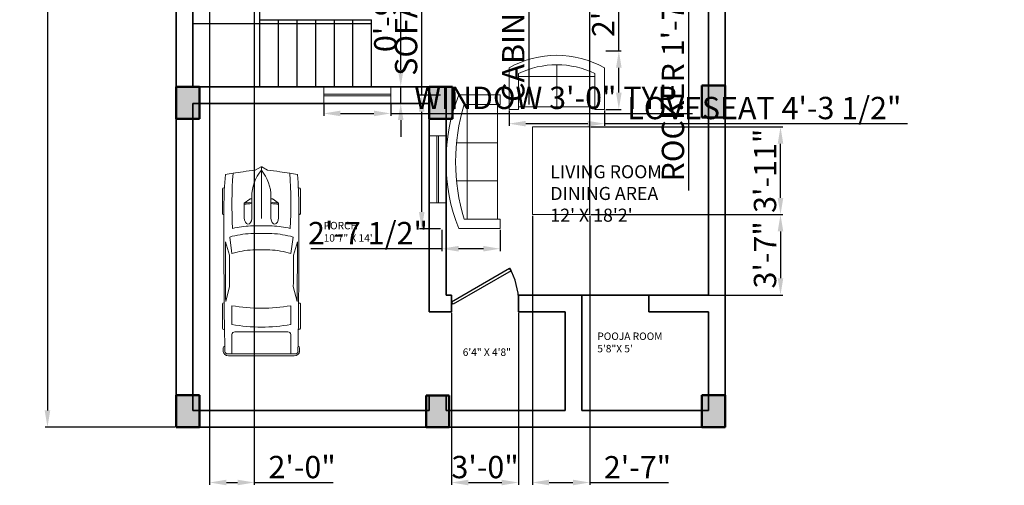
# Model space of a CAD drawing. Units: inches. Extents: x 1132 to 1713, y 3115 to 3781.
# Tile 1 of 4: x 1184 to 1713, y 3115 to 3365. Entities that reach past the tile are written whole.
import ezdxf

# ---------------------------------------------------------------- set-up
doc = ezdxf.new("R2010")
doc.units = ezdxf.units.IN
for name, color, linetype, lineweight in [('A-ANNO-DIMS', 2, 'Continuous', 18), ('A-AREA-IDEN', 7, 'Continuous', 18), ('A-COLS', 1, 'Continuous', 50), ('A-COLS-PATT', 252, 'Continuous', 13), ('A-DOOR', 3, 'Continuous', 25), ('A-FLOR-STRS', 7, 'Continuous', 25), ('A-FURN', 8, 'Continuous', 18), ('A-GLAZ', 4, 'Continuous', 18), ('A-SITE-VEHS', 9, 'Continuous', 13), ('A-WALL', 7, 'Continuous', 35)]:
    doc.layers.add(name, color=color, linetype=linetype, lineweight=lineweight)
doc.styles.get("Standard").update_dxf_attribs({"font": 'arial.ttf'})
doc.dimstyles.new('ISO-25', dxfattribs={"dimtxt": 12, "dimasz": 9, "dimexe": 1.25, "dimexo": 0.625, "dimtad": 1, "dimdec": 0, "dimrnd": 2, "dimlunit": 3, "dimtxsty": 'Standard', "dimcen": 2.5, "dimadec": 0, "dimazin": 0, "dimtfac": 1, "dimtdec": 0, "dimtmove": 0, "dimatfit": 3, "dimfxl": 1, "dimarcsym": 0})

# ---------------------------------------------------------------- blocks, each defined once
blk = doc.blocks.new('*U2')
for p, q in [((0, 0), (0, -6)), ((40, 0), (40, -6))]:
    blk.add_line(p, q)
blk.add_lwpolyline([(0, 0), (34.64, 20), (35.52, 18.48), (0.87, -1.52)], close=True)
blk.add_arc((0, 0), 40, 0, 30)
blk = doc.blocks.new('Sofa - Roundback Loveseat 5 ft.')
for p, q in [((0, -32.44198), (0, -5.99998)), ((-24, -33.99998), (-24, -11.46958)), ((24.00004, -33.99998), (24.00004, -11.46958)), ((-23.9998, -13.38178), (23.99986, -13.38178)), ((-24, -32.44198), (24.00004, -32.44198))]:
    blk.add_line(p, q)
for points in [[(-24, -33.99998), (-30, -33.99998), (-30, -7.99998)], [(30.00004, -7.99998), (30.00004, -33.99998), (24.00004, -33.99998)]]:
    blk.add_lwpolyline(points)
for centre, radius, start, end in [((0, -60.24998), 60.24998, 60.13715, 119.8628), ((0, -61.38438), 55.38444, 64.32083, 115.6792)]:
    blk.add_arc(centre, radius, start, end)
blk = doc.blocks.new('Sofa - Roundback 7 ft.')
for p, q in [((-36.000027, -34), (-36.000027, -11.4696)), ((-12.00002, -32.4421), (-12.00003, -6.5971)), ((11.99997, -32.4421), (11.99998, -6.5971)), ((35.99998, -34), (35.99998, -11.4696)), ((-35.999844, -13.3819), (35.9998, -13.3819)), ((-36.000027, -32.4421), (35.99998, -32.4421))]:
    blk.add_line(p, q)
for points in [[(-36.000027, -34), (-42.000027, -34), (-42.000027, -8)], [(41.99998, -8), (41.99998, -34), (35.99998, -34)]]:
    blk.add_lwpolyline(points)
for centre, radius, start, end in [((0, -114.25), 114.25, 68.43141, 111.5686), ((-0.00001, -127.1968), 121.1968, 72.72033, 107.2797)]:
    blk.add_arc(centre, radius, start, end)
blk = doc.blocks.new('*U17')
for p, q in [((536, 950), (536, 936)), ((1182, 988), (568, 988)), ((1214, 950), (1214, 950)), ((1779, 801), (2195, 746)), ((2235, 810), (1899, 912)), ((3412, 904), (3030, 807)), ((3440, 942), (3440, 950)), ((3472, 988), (4087, 988)), ((4119, 950), (4119, 934)), ((4736, -851), (4736, 851)), ((4785, -832), (4785, 832)), ((3516, 746), (3994, 746)), ((4179, 670), (4179, -670)), ((4736, 746), (4242, 746)), ((816, 241), (816, 283)), ((820, 295), (918, 436)), ((918, 436), (1294, 436)), ((1496, -274), (1496, 274)), ((1690, -267), (1690, 267)), ((4736, -267), (4736, 267)), ((83, 156), (3, 10)), ((756, 241), (1313, 241)), ((2102, 216), (2102, -216)), ((0, 0), (1313, 0)), ((3, -10), (83, -156)), ((756, -241), (1313, -241)), ((816, -241), (816, -283)), ((820, -295), (918, -436)), ((918, -436), (1294, -436)), ((2195, -746), (1779, -801)), ((3994, -746), (3516, -746)), ((4242, -746), (4736, -746)), ((536, -950), (536, -936)), ((1182, -988), (568, -988)), ((1214, -950), (1214, -950)), ((2235, -810), (1899, -912)), ((3412, -904), (3030, -807)), ((3440, -942), (3440, -950)), ((3472, -988), (4087, -988)), ((4119, -950), (4119, -934))]:
    blk.add_line(p, q)
for centre, major_axis, ratio, start_param, end_param in [((6757, -699), (0, 7958), 0.842304, 1.367076, 1.39176), ((952, -15087), (0, -15833), 0.842304, 3.096046, 3.200911), ((1046, -12468), (0, 13417), 0.842304, 0.00281, 0.075598), ((568, 950), (0, -37.6), 0.842304, 3.141593, 4.712389), ((1638, -268113), (0, 269063), 0.842304, -0.013397, 0.002797), ((1182, 950), (0, 37.6), 0.842304, -1.570796, 0), ((3436, 137), (0, 2077), 0.842304, 1.245306, 1.50788), ((1638, -268113), (0, -269025), 0.842304, 3.133765, 3.140441), ((2433, -93125), (0, -93935), 0.842304, 3.134049, 3.144098), ((3472, 950), (0, -37.6), 0.842304, 3.141593, 4.712389), ((4087, 950), (0, 37.6), 0.842304, -1.570796, 0), ((4588, 910), (0, 56.4), 0.842304, -0.013017, 1.249894), ((1638, -268131), (0, 269121), 0.842304, -0.013397, -0.013017), ((4673, 851), (0, -75.2), 0.842304, 1.570796, 3.128196), ((4673, 832), (0, -133), 0.842304, 1.570796, 3.128196), ((6583, -699), (0, -7755), 0.842304, 4.528606, 4.561838), ((3414, 137), (0, -2280), 0.842304, 4.449482, 4.652344), ((3800, 71), (0, -2021), 0.842304, 4.372215, 4.640744), ((434, 0), (0, 3734), 0.842304, 4.511394, 4.913384), ((912, 0), (0, 3734), 0.842304, 4.511394, 4.913384), ((4242, 670), (0, 75.2), 0.842304, 0, 1.570796), ((-5194, 1331), (0, -6374), 0.842304, 1.385369, 1.434372), ((832, 283), (0, 18.8), 0.842304, 0.879714, 1.570796), ((331, 432), (0, 696), 0.842304, 4.435146, 4.718221), ((361, 432), (0, 696), 0.842304, 4.435146, 4.718221), ((1290, 339), (161, -9), 0.603834, -1.395552, 1.581315), ((16, 0), (0, -18.8), 0.842304, 4.131459, 5.293319), ((756, -1185), (0, 1427), 0.842304, 0, 0.590319), ((-5194, -1331), (0, 6374), 0.842304, -1.434372, -1.385369), ((756, 1185), (0, 1427), 0.842304, 2.551274, 3.141593), ((331, -432), (0, -696), 0.842304, 1.564964, 1.848039), ((361, -432), (0, -696), 0.842304, 1.564964, 1.848039), ((3800, -71), (0, -2021), 0.842304, -1.499151, -1.230623), ((6583, 699), (0, 7755), 0.842304, 1.721348, 1.754579), ((832, -283), (0, -18.8), 0.842304, 4.712389, 5.403472), ((3414, -137), (0, -2280), 0.842304, -1.510751, -1.307889), ((3436, -137), (0, -2077), 0.842304, -1.50788, -1.245306), ((6757, 699), (0, 7958), 0.842304, 1.749832, 1.774517), ((952, 15087), (0, -15833), 0.842304, -0.059319, 0.045547), ((4242, -670), (0, -75.2), 0.842304, 4.712389, 6.283185), ((1046, 12468), (0, -13417), 0.842304, -0.075598, -0.00281), ((568, -950), (0, 37.6), 0.842304, 1.570796, 3.141593), ((1638, 268113), (0, 269063), 0.842304, 3.138796, 3.15499), ((1182, -950), (0, -37.6), 0.842304, 0, 1.570796), ((1638, 268113), (0, -269025), 0.842304, 0.001152, 0.007828), ((2433, 93125), (0, -93935), 0.842304, -0.002505, 0.007544), ((3472, -950), (0, -37.6), 0.842304, -1.570796, 0), ((4087, -950), (0, 37.6), 0.842304, 3.141593, 4.712389), ((4588, -910), (0, -56.4), 0.842304, -1.249894, 0.013017), ((1638, 268131), (0, 269121), 0.842304, 3.15461, 3.15499), ((4673, -851), (0, 75.2), 0.842304, 3.15499, 4.712389), ((4673, -832), (0, -133), 0.842304, 0.013397, 1.570796)]:
    blk.add_ellipse(centre, major_axis=major_axis, ratio=ratio, start_param=start_param, end_param=end_param)
at = {"extrusion": (0, 0, -1)}
blk.add_ellipse((1290, -339), major_axis=(161, 9), ratio=0.603834, start_param=-1.395552, end_param=1.581315, dxfattribs=at)
blk = doc.blocks.new('*D18')
at = {"layer": 'A-ANNO-DIMS', "color": 0, "lineweight": -2, "transparency": 16777216}
for p, q in [((1267.53, 3670.88), (1197.76, 3670.88)), ((1199.01, 3661.88), (1199.01, 3154.88)), ((1267.53, 3145.88), (1197.76, 3145.88))]:
    blk.add_line(p, q, dxfattribs=at)
at = {"layer": 'A-ANNO-DIMS', "color": 0, "transparency": 16777216}
for points in [[(1197.51, 3661.88), (1200.51, 3661.88), (1199.01, 3670.88)], [(1197.51, 3154.88), (1200.51, 3154.88), (1199.01, 3145.88)]]:
    blk.add_solid(points, dxfattribs=at)
at = {"layer": 'Defpoints', "color": 0, "transparency": 16777216}
for p in [(1268.16, 3670.88), (1199.01, 3145.88), (1268.16, 3145.88)]:
    blk.add_point(p, dxfattribs=at)
at = {"layer": 'A-ANNO-DIMS', "color": 0, "transparency": 16777216, "insert": (1192.25, 3408.38), "char_height": 12, "attachment_point": 5, "rotation": 90}
blk.add_mtext('43\'-8"', dxfattribs=at)
blk = doc.blocks.new('WIN-36IN')
for p, q in [((-36, 0), (-36, 9)), ((-36, 9), (0, 9)), ((0, 9), (0, 0)), ((-36, 5), (0, 5)), ((0, 4), (-36, 4)), ((0, 0), (-36, 0))]:
    blk.add_line(p, q)
blk = doc.blocks.new('*D24')
at = {"layer": 'A-ANNO-DIMS', "color": 0, "lineweight": -2, "transparency": 16777216}
for p, q in [((1543.52, 3469.28), (1543.52, 3478.28)), ((1541.29, 3460.28), (1544.77, 3460.28)), ((1543.52, 3460.28), (1543.52, 3441.25)), ((1541.29, 3441.25), (1544.77, 3441.25)), ((1543.52, 3432.25), (1543.52, 3273.09))]:
    blk.add_line(p, q, dxfattribs=at)
at = {"layer": 'A-ANNO-DIMS', "color": 0, "transparency": 16777216}
for points in [[(1542.02, 3469.28), (1545.02, 3469.28), (1543.52, 3460.28)], [(1542.02, 3432.25), (1545.02, 3432.25), (1543.52, 3441.25)]]:
    blk.add_solid(points, dxfattribs=at)
at = {"layer": 'Defpoints', "color": 0, "transparency": 16777216}
for p in [(1540.66, 3460.28), (1540.66, 3441.25), (1543.52, 3441.25)]:
    blk.add_point(p, dxfattribs=at)
at = {"layer": 'A-ANNO-DIMS', "color": 0, "transparency": 16777216, "insert": (1536.68, 3348.17), "char_height": 12, "attachment_point": 5, "rotation": 90}
blk.add_mtext('ROCKER 1\'-7" TYP.', dxfattribs=at)
blk = doc.blocks.new('*D26')
at = {"layer": 'A-ANNO-DIMS', "color": 0, "lineweight": -2, "transparency": 16777216}
for p, q in [((1347.43, 3319.25), (1347.43, 3313.23)), ((1383.43, 3319.25), (1383.43, 3313.23)), ((1356.43, 3314.48), (1374.43, 3314.48)), ((1383.43, 3314.48), (1545.53, 3314.48))]:
    blk.add_line(p, q, dxfattribs=at)
at = {"layer": 'A-ANNO-DIMS', "color": 0, "transparency": 16777216}
for points in [[(1356.43, 3315.98), (1356.43, 3312.98), (1347.43, 3314.48)], [(1374.43, 3315.98), (1374.43, 3312.98), (1383.43, 3314.48)]]:
    blk.add_solid(points, dxfattribs=at)
at = {"layer": 'Defpoints', "color": 0, "transparency": 16777216}
for p in [(1347.43, 3319.88), (1383.43, 3319.88), (1383.43, 3314.48)]:
    blk.add_point(p, dxfattribs=at)
at = {"layer": 'A-ANNO-DIMS', "color": 0, "transparency": 16777216, "insert": (1468.98, 3321.31), "char_height": 12, "attachment_point": 5}
blk.add_mtext('WINDOW 3\'-0" TYP.', dxfattribs=at)
blk = doc.blocks.new('*D27')
at = {"layer": 'A-ANNO-DIMS', "color": 0, "lineweight": -2, "transparency": 16777216}
for p, q in [((1388.83, 3337.88), (1388.83, 3421.27)), ((1384.06, 3328.88), (1390.08, 3328.88)), ((1388.83, 3319.88), (1388.83, 3328.88)), ((1384.06, 3319.88), (1390.08, 3319.88)), ((1388.83, 3310.88), (1388.83, 3301.88))]:
    blk.add_line(p, q, dxfattribs=at)
at = {"layer": 'A-ANNO-DIMS', "color": 0, "transparency": 16777216}
for points in [[(1387.33, 3337.88), (1390.33, 3337.88), (1388.83, 3328.88)], [(1387.33, 3310.88), (1390.33, 3310.88), (1388.83, 3319.88)]]:
    blk.add_solid(points, dxfattribs=at)
at = {"layer": 'Defpoints', "color": 0, "transparency": 16777216}
for p in [(1383.43, 3328.88), (1388.83, 3328.88), (1383.43, 3319.88)]:
    blk.add_point(p, dxfattribs=at)
at = {"layer": 'A-ANNO-DIMS', "color": 0, "transparency": 16777216, "insert": (1382.08, 3384.07), "char_height": 12, "attachment_point": 5, "rotation": 90}
blk.add_mtext('0\'-9" TYP.', dxfattribs=at)
blk = doc.blocks.new('*D30')
at = {"layer": 'A-ANNO-DIMS', "color": 0, "lineweight": -2, "transparency": 16777216}
for p, q in [((1447.03, 3316.07), (1447.03, 3307.75)), ((1498.35, 3316.07), (1498.35, 3307.75)), ((1456.03, 3309), (1489.35, 3309)), ((1498.35, 3309), (1661.09, 3309))]:
    blk.add_line(p, q, dxfattribs=at)
at = {"layer": 'A-ANNO-DIMS', "color": 0, "transparency": 16777216}
for points in [[(1456.03, 3310.5), (1456.03, 3307.5), (1447.03, 3309)], [(1489.35, 3310.5), (1489.35, 3307.5), (1498.35, 3309)]]:
    blk.add_solid(points, dxfattribs=at)
at = {"layer": 'Defpoints', "color": 0, "transparency": 16777216}
for p in [(1447.03, 3316.7), (1498.35, 3316.7), (1498.35, 3309)]:
    blk.add_point(p, dxfattribs=at)
at = {"layer": 'A-ANNO-DIMS', "color": 0, "transparency": 16777216, "insert": (1584.22, 3315.84), "char_height": 12, "attachment_point": 5}
blk.add_mtext('LOVESEAT 4\'-3 1/2"', dxfattribs=at)
blk = doc.blocks.new('*D31')
at = {"layer": 'A-ANNO-DIMS', "color": 0, "lineweight": -2, "transparency": 16777216}
for p, q in [((1506.04, 3348.05), (1506.04, 3418.37)), ((1498.97, 3348.05), (1507.29, 3348.05)), ((1506.04, 3325.7), (1506.04, 3339.05)), ((1498.97, 3316.7), (1507.29, 3316.7))]:
    blk.add_line(p, q, dxfattribs=at)
at = {"layer": 'A-ANNO-DIMS', "color": 0, "transparency": 16777216}
for points in [[(1504.54, 3339.05), (1507.54, 3339.05), (1506.04, 3348.05)], [(1504.54, 3325.7), (1507.54, 3325.7), (1506.04, 3316.7)]]:
    blk.add_solid(points, dxfattribs=at)
at = {"layer": 'Defpoints', "color": 0, "transparency": 16777216}
for p in [(1498.35, 3348.05), (1506.04, 3348.05), (1498.35, 3316.7)]:
    blk.add_point(p, dxfattribs=at)
at = {"layer": 'A-ANNO-DIMS', "color": 0, "transparency": 16777216, "insert": (1499.21, 3387.71), "char_height": 12, "attachment_point": 5, "rotation": 90}
blk.add_mtext('2\'-7 1/2"', dxfattribs=at)
blk = doc.blocks.new('*D32')
at = {"layer": 'A-ANNO-DIMS', "color": 0, "lineweight": -2, "transparency": 16777216}
for p, q in [((1400.1, 3324.4), (1400.1, 3416.8)), ((1410.25, 3324.4), (1398.85, 3324.4)), ((1400.1, 3261.57), (1400.1, 3315.4)), ((1410.25, 3252.57), (1398.85, 3252.57))]:
    blk.add_line(p, q, dxfattribs=at)
at = {"layer": 'A-ANNO-DIMS', "color": 0, "transparency": 16777216}
for points in [[(1398.6, 3315.4), (1401.6, 3315.4), (1400.1, 3324.4)], [(1398.6, 3261.57), (1401.6, 3261.57), (1400.1, 3252.57)]]:
    blk.add_solid(points, dxfattribs=at)
at = {"layer": 'Defpoints', "color": 0, "transparency": 16777216}
for p in [(1400.1, 3324.4), (1410.88, 3324.4), (1410.88, 3252.57)]:
    blk.add_point(p, dxfattribs=at)
at = {"layer": 'A-ANNO-DIMS', "color": 0, "transparency": 16777216, "insert": (1393.27, 3375.1), "char_height": 12, "attachment_point": 5, "rotation": 90}
blk.add_mtext('SOFA 6\'-0"', dxfattribs=at)
blk = doc.blocks.new('*D33')
at = {"layer": 'A-ANNO-DIMS', "color": 0, "lineweight": -2, "transparency": 16777216}
for p, q in [((1410.88, 3251.94), (1410.88, 3240.54)), ((1442.24, 3251.94), (1442.24, 3240.54)), ((1410.88, 3241.79), (1340.56, 3241.79)), ((1433.24, 3241.79), (1419.88, 3241.79))]:
    blk.add_line(p, q, dxfattribs=at)
at = {"layer": 'A-ANNO-DIMS', "color": 0, "transparency": 16777216}
for points in [[(1419.88, 3243.29), (1419.88, 3240.29), (1410.88, 3241.79)], [(1433.24, 3243.29), (1433.24, 3240.29), (1442.24, 3241.79)]]:
    blk.add_solid(points, dxfattribs=at)
at = {"layer": 'Defpoints', "color": 0, "transparency": 16777216}
for p in [(1410.88, 3252.57), (1442.24, 3252.57), (1410.88, 3241.79)]:
    blk.add_point(p, dxfattribs=at)
at = {"layer": 'A-ANNO-DIMS', "color": 0, "transparency": 16777216, "insert": (1371.22, 3248.62), "char_height": 12, "attachment_point": 5}
blk.add_mtext('2\'-7 1/2"', dxfattribs=at)
blk = doc.blocks.new('*D40')
at = {"layer": 'A-ANNO-DIMS', "color": 0, "lineweight": -2, "transparency": 16777216}
for p, q in [((1452.73, 3503.82), (1458.96, 3503.82)), ((1457.71, 3494.82), (1457.71, 3475.51)), ((1452.73, 3466.51), (1458.96, 3466.51)), ((1457.71, 3466.51), (1457.71, 3319.22))]:
    blk.add_line(p, q, dxfattribs=at)
at = {"layer": 'A-ANNO-DIMS', "color": 0, "transparency": 16777216}
for points in [[(1456.21, 3494.82), (1459.21, 3494.82), (1457.71, 3503.82)], [(1456.21, 3475.51), (1459.21, 3475.51), (1457.71, 3466.51)]]:
    blk.add_solid(points, dxfattribs=at)
at = {"layer": 'Defpoints', "color": 0, "transparency": 16777216}
for p in [(1452.11, 3503.82), (1452.11, 3466.51), (1457.71, 3466.51)]:
    blk.add_point(p, dxfattribs=at)
at = {"layer": 'A-ANNO-DIMS', "color": 0, "transparency": 16777216, "insert": (1450.87, 3388.36), "char_height": 12, "attachment_point": 5, "rotation": 90}
blk.add_mtext('CABINET 3\'-1 1/2"', dxfattribs=at)
blk = doc.blocks.new('*D44')
at = {"layer": 'A-ANNO-DIMS', "color": 0, "lineweight": -2, "transparency": 16777216}
for p, q in [((1463.04, 3385.85), (1463.04, 3374.62)), ((1533.74, 3385.85), (1533.74, 3374.62)), ((1472.04, 3375.87), (1524.74, 3375.87)), ((1533.74, 3375.87), (1713.17, 3375.87))]:
    blk.add_line(p, q, dxfattribs=at)
at = {"layer": 'A-ANNO-DIMS', "color": 0, "transparency": 16777216}
for points in [[(1472.04, 3377.37), (1472.04, 3374.37), (1463.04, 3375.87)], [(1524.74, 3377.37), (1524.74, 3374.37), (1533.74, 3375.87)]]:
    blk.add_solid(points, dxfattribs=at)
at = {"layer": 'Defpoints', "color": 0, "transparency": 16777216}
for p in [(1463.04, 3386.48), (1533.74, 3386.48), (1533.74, 3375.87)]:
    blk.add_point(p, dxfattribs=at)
at = {"layer": 'A-ANNO-DIMS', "color": 0, "transparency": 16777216, "insert": (1627.96, 3382.7), "char_height": 12, "attachment_point": 5}
blk.add_mtext('DINING SET 5\'-10 1/2"', dxfattribs=at)
blk = doc.blocks.new('*D46')
at = {"layer": 'A-ANNO-DIMS', "color": 0, "lineweight": -2, "transparency": 16777216}
for p, q in [((1277.16, 3363.5), (1277.16, 3701.81)), ((1286.16, 3700.56), (1304.16, 3700.56)), ((1313.16, 3365.5), (1313.16, 3701.81))]:
    blk.add_line(p, q, dxfattribs=at)
at = {"layer": 'A-ANNO-DIMS', "color": 0, "transparency": 16777216}
for points in [[(1286.16, 3702.06), (1286.16, 3699.06), (1277.16, 3700.56)], [(1304.16, 3702.06), (1304.16, 3699.06), (1313.16, 3700.56)]]:
    blk.add_solid(points, dxfattribs=at)
at = {"layer": 'Defpoints', "color": 0, "transparency": 16777216}
for p in [(1313.16, 3700.56), (1277.16, 3362.88), (1313.16, 3364.88)]:
    blk.add_point(p, dxfattribs=at)
at = {"layer": 'A-ANNO-DIMS', "color": 0, "transparency": 16777216, "insert": (1295.16, 3707.32), "char_height": 12, "attachment_point": 5}
blk.add_mtext('3\'-0"', dxfattribs=at)
blk = doc.blocks.new('*D48')
at = {"layer": 'A-ANNO-DIMS', "color": 0, "lineweight": -2, "transparency": 16777216}
for p, q in [((1491, 3307.23), (1594.15, 3307.23)), ((1592.9, 3269.12), (1592.9, 3298.23)), ((1491, 3260.12), (1594.15, 3260.12))]:
    blk.add_line(p, q, dxfattribs=at)
at = {"layer": 'A-ANNO-DIMS', "color": 0, "transparency": 16777216}
for points in [[(1591.4, 3298.23), (1594.4, 3298.23), (1592.9, 3307.23)], [(1591.4, 3269.12), (1594.4, 3269.12), (1592.9, 3260.12)]]:
    blk.add_solid(points, dxfattribs=at)
at = {"layer": 'Defpoints', "color": 0, "transparency": 16777216}
for p in [(1490.38, 3307.23), (1592.9, 3307.23), (1490.38, 3260.12)]:
    blk.add_point(p, dxfattribs=at)
at = {"layer": 'A-ANNO-DIMS', "color": 0, "transparency": 16777216, "insert": (1586.14, 3283.67), "char_height": 12, "attachment_point": 5, "rotation": 90}
blk.add_mtext('3\'-11"', dxfattribs=at)
blk = doc.blocks.new('*D49')
at = {"layer": 'A-ANNO-DIMS', "color": 0, "lineweight": -2, "transparency": 16777216}
for p, q in [((1459.58, 3259.49), (1459.58, 3114.9)), ((1490.38, 3259.49), (1490.38, 3114.9)), ((1468.58, 3116.15), (1481.38, 3116.15)), ((1490.38, 3116.15), (1532.73, 3116.15))]:
    blk.add_line(p, q, dxfattribs=at)
at = {"layer": 'A-ANNO-DIMS', "color": 0, "transparency": 16777216}
for points in [[(1468.58, 3117.65), (1468.58, 3114.65), (1459.58, 3116.15)], [(1481.38, 3117.65), (1481.38, 3114.65), (1490.38, 3116.15)]]:
    blk.add_solid(points, dxfattribs=at)
at = {"layer": 'Defpoints', "color": 0, "transparency": 16777216}
for p in [(1459.58, 3260.12), (1490.38, 3260.12), (1490.38, 3116.15)]:
    blk.add_point(p, dxfattribs=at)
at = {"layer": 'A-ANNO-DIMS', "color": 0, "transparency": 16777216, "insert": (1516.05, 3122.8), "char_height": 12, "attachment_point": 5}
blk.add_mtext('2\'-7"', dxfattribs=at)
blk = doc.blocks.new('*D50')
at = {"layer": 'A-ANNO-DIMS', "color": 0, "lineweight": -2, "transparency": 16777216}
for p, q in [((1490.38, 3260.74), (1490.38, 3701.81)), ((1499.38, 3700.56), (1545.16, 3700.56)), ((1554.16, 3217.5), (1554.16, 3701.81))]:
    blk.add_line(p, q, dxfattribs=at)
at = {"layer": 'A-ANNO-DIMS', "color": 0, "transparency": 16777216}
for points in [[(1499.38, 3702.06), (1499.38, 3699.06), (1490.38, 3700.56)], [(1545.16, 3702.06), (1545.16, 3699.06), (1554.16, 3700.56)]]:
    blk.add_solid(points, dxfattribs=at)
at = {"layer": 'Defpoints', "color": 0, "transparency": 16777216}
for p in [(1554.16, 3700.56), (1490.38, 3260.12), (1554.16, 3216.88)]:
    blk.add_point(p, dxfattribs=at)
at = {"layer": 'A-ANNO-DIMS', "color": 0, "transparency": 16777216, "insert": (1522.27, 3707.29), "char_height": 12, "attachment_point": 5}
blk.add_mtext('5\'-4"', dxfattribs=at)
blk = doc.blocks.new('*D51')
at = {"layer": 'A-ANNO-DIMS', "color": 0, "lineweight": -2, "transparency": 16777216}
for p, q in [((1491, 3260.12), (1594.15, 3260.12)), ((1592.9, 3251.12), (1592.9, 3225.88)), ((1486.78, 3216.88), (1594.15, 3216.88))]:
    blk.add_line(p, q, dxfattribs=at)
at = {"layer": 'A-ANNO-DIMS', "color": 0, "transparency": 16777216}
for points in [[(1591.4, 3251.12), (1594.4, 3251.12), (1592.9, 3260.12)], [(1591.4, 3225.88), (1594.4, 3225.88), (1592.9, 3216.88)]]:
    blk.add_solid(points, dxfattribs=at)
at = {"layer": 'Defpoints', "color": 0, "transparency": 16777216}
for p in [(1490.38, 3260.12), (1486.16, 3216.88), (1592.9, 3216.88)]:
    blk.add_point(p, dxfattribs=at)
at = {"layer": 'A-ANNO-DIMS', "color": 0, "transparency": 16777216, "insert": (1586.14, 3238.5), "char_height": 12, "attachment_point": 5, "rotation": 90}
blk.add_mtext('3\'-7"', dxfattribs=at)
blk = doc.blocks.new('*D52')
at = {"layer": 'A-ANNO-DIMS', "color": 0, "lineweight": -2, "transparency": 16777216}
for p, q in [((1416.16, 3207.25), (1416.16, 3114.9)), ((1452.16, 3207.25), (1452.16, 3114.9)), ((1425.16, 3116.15), (1443.16, 3116.15))]:
    blk.add_line(p, q, dxfattribs=at)
at = {"layer": 'A-ANNO-DIMS', "color": 0, "transparency": 16777216}
for points in [[(1425.16, 3117.65), (1425.16, 3114.65), (1416.16, 3116.15)], [(1443.16, 3117.65), (1443.16, 3114.65), (1452.16, 3116.15)]]:
    blk.add_solid(points, dxfattribs=at)
at = {"layer": 'Defpoints', "color": 0, "transparency": 16777216}
for p in [(1416.16, 3207.88), (1452.16, 3207.88), (1452.16, 3116.15)]:
    blk.add_point(p, dxfattribs=at)
at = {"layer": 'A-ANNO-DIMS', "color": 0, "transparency": 16777216, "insert": (1434.16, 3122.9), "char_height": 12, "attachment_point": 5}
blk.add_mtext('3\'-0"', dxfattribs=at)
blk = doc.blocks.new('*D53')
at = {"layer": 'A-ANNO-DIMS', "color": 0, "lineweight": -2, "transparency": 16777216}
for p, q in [((1286.16, 3582.14), (1286.16, 3114.9)), ((1310.16, 3582.25), (1310.16, 3114.9)), ((1295.16, 3116.15), (1301.16, 3116.15)), ((1310.16, 3116.15), (1352.51, 3116.15))]:
    blk.add_line(p, q, dxfattribs=at)
at = {"layer": 'A-ANNO-DIMS', "color": 0, "transparency": 16777216}
for points in [[(1295.16, 3117.65), (1295.16, 3114.65), (1286.16, 3116.15)], [(1301.16, 3117.65), (1301.16, 3114.65), (1310.16, 3116.15)]]:
    blk.add_solid(points, dxfattribs=at)
at = {"layer": 'Defpoints', "color": 0, "transparency": 16777216}
for p in [(1286.16, 3582.77), (1310.16, 3582.88), (1310.16, 3116.15)]:
    blk.add_point(p, dxfattribs=at)
at = {"layer": 'A-ANNO-DIMS', "color": 0, "transparency": 16777216, "insert": (1335.84, 3122.9), "char_height": 12, "attachment_point": 5}
blk.add_mtext('2\'-0"', dxfattribs=at)

msp = doc.modelspace()

# ---------------------------------------------------------------- hatches: boundary and pattern name
at = {"layer": 'A-COLS-PATT'}
h = msp.add_hatch(color=256, dxfattribs=at)
h.dxf.hatch_style = 1
h.paths.add_polyline_path([(1268.16, 3311.61), (1277.16, 3311.61), (1277.16, 3319.88), (1280.66, 3319.88), (1280.66, 3328.79), (1268.16, 3328.79)])
h = msp.add_hatch(color=256, dxfattribs=at)
h.dxf.hatch_style = 1
h.paths.add_polyline_path([(1413.16, 3328.79), (1404.16, 3328.79), (1404.16, 3311.61), (1413.16, 3311.61), (1413.16, 3319.88)])
h = msp.add_hatch(color=256, dxfattribs=at)
h.dxf.hatch_style = 1
h.paths.add_polyline_path([(1413.16, 3311.61), (1416.66, 3311.61), (1416.66, 3328.79), (1413.16, 3328.79), (1413.16, 3319.88)])
h = msp.add_hatch(color=256, dxfattribs=at)
h.dxf.hatch_style = 1
h.paths.add_polyline_path([(1550.69, 3312.4), (1554.16, 3312.4), (1554.16, 3329.57), (1550.69, 3329.57)])
h = msp.add_hatch(color=256, dxfattribs=at)
h.dxf.hatch_style = 1
h.paths.add_polyline_path([(1554.16, 3312.4), (1563.16, 3312.4), (1563.16, 3329.57), (1554.16, 3329.57)])
h = msp.add_hatch(color=256, dxfattribs=at)
h.dxf.hatch_style = 1
h.paths.add_polyline_path([(1277.16, 3311.61), (1280.66, 3311.61), (1280.66, 3319.88), (1277.16, 3319.88)])
h = msp.add_hatch(color=256, dxfattribs=at)
h.dxf.hatch_style = 1
h.paths.add_polyline_path([(1280.66, 3145.88), (1280.66, 3154.88), (1277.16, 3154.88), (1277.16, 3163.05), (1268.16, 3163.05), (1268.16, 3145.88)])
h = msp.add_hatch(color=256, dxfattribs=at)
h.dxf.hatch_style = 1
h.paths.add_polyline_path([(1280.66, 3163.05), (1277.16, 3163.05), (1277.16, 3154.88), (1280.66, 3154.88)])
h = msp.add_hatch(color=256, dxfattribs=at)
h.dxf.hatch_style = 1
h.paths.add_polyline_path([(1404.16, 3154.88), (1402.42, 3154.88), (1402.42, 3145.88), (1414.92, 3145.88), (1414.92, 3154.88), (1413.16, 3154.88), (1413.16, 3162.99), (1404.16, 3162.99)])
h = msp.add_hatch(color=256, dxfattribs=at)
h.dxf.hatch_style = 1
h.paths.add_polyline_path([(1404.16, 3162.99), (1402.42, 3162.99), (1402.42, 3154.88), (1404.16, 3154.88)])
h = msp.add_hatch(color=256, dxfattribs=at)
h.dxf.hatch_style = 1
h.paths.add_polyline_path([(1414.92, 3162.99), (1413.16, 3162.99), (1413.16, 3154.88), (1414.92, 3154.88)])
h = msp.add_hatch(color=256, dxfattribs=at)
h.dxf.hatch_style = 1
h.paths.add_polyline_path([(1550.69, 3154.88), (1554.16, 3154.88), (1554.16, 3163.11), (1550.69, 3163.11)])
h = msp.add_hatch(color=256, dxfattribs=at)
h.dxf.hatch_style = 1
h.paths.add_polyline_path([(1550.69, 3154.88), (1550.69, 3145.93), (1563.16, 3145.93), (1563.16, 3163.11), (1554.16, 3163.11), (1554.16, 3154.88)])

# ---------------------------------------------------------------- linework, layer by layer
at = {"layer": 'A-COLS'}
for p, q in [((1268.16, 3328.79), (1268.16, 3319.79)), ((1268.16, 3328.79), (1280.66, 3328.79)), ((1268.16, 3311.61), (1268.16, 3328.79)), ((1280.66, 3328.79), (1280.66, 3311.61)), ((1404.16, 3328.79), (1416.66, 3328.79)), ((1404.16, 3311.61), (1404.16, 3328.79)), ((1416.66, 3328.79), (1416.66, 3311.61)), ((1550.69, 3329.57), (1563.19, 3329.57)), ((1550.69, 3312.4), (1550.69, 3329.57)), ((1563.19, 3329.57), (1563.19, 3312.4)), ((1268.16, 3321.75), (1268.16, 3312.75)), ((1563.19, 3312.4), (1550.69, 3312.4)), ((1280.66, 3311.61), (1268.16, 3311.61)), ((1416.66, 3311.61), (1404.16, 3311.61)), ((1268.16, 3163.05), (1280.66, 3163.05)), ((1268.16, 3145.88), (1268.16, 3163.05)), ((1280.66, 3163.05), (1280.66, 3145.88)), ((1402.42, 3162.99), (1414.92, 3162.99)), ((1402.42, 3145.82), (1402.42, 3162.99)), ((1414.92, 3162.99), (1414.92, 3145.82)), ((1550.69, 3163.11), (1563.19, 3163.11)), ((1550.69, 3145.93), (1550.69, 3163.11)), ((1563.19, 3163.11), (1563.19, 3145.93)), ((1280.66, 3145.88), (1268.16, 3145.88)), ((1414.92, 3145.82), (1402.42, 3145.82)), ((1563.19, 3145.93), (1550.69, 3145.93))]:
    msp.add_line(p, q, dxfattribs=at)
at = {"layer": 'A-FLOR-STRS'}
for p, q in [((1313.16, 3328.88), (1313.16, 3434.88)), ((1277.16, 3362.88), (1373.16, 3362.88)), ((1313.16, 3364.88), (1373.16, 3364.88)), ((1323.16, 3328.88), (1323.16, 3364.88)), ((1333.16, 3328.88), (1333.16, 3364.88)), ((1343.16, 3328.88), (1343.16, 3364.88)), ((1353.16, 3328.88), (1353.16, 3364.88)), ((1363.16, 3328.88), (1363.16, 3364.88)), ((1373.16, 3328.88), (1373.16, 3364.88))]:
    msp.add_line(p, q, dxfattribs=at)
at = {"layer": 'A-FURN'}
msp.add_lwpolyline([(1459.58, 3307.23), (1490.38, 3307.23), (1490.38, 3260.12), (1459.58, 3260.12)], close=True, dxfattribs=at)
at = {"layer": 'A-WALL'}
for p, q in [((1277.16, 3328.88), (1277.16, 3434.88)), ((1554.16, 3434.88), (1554.16, 3216.88)), ((1277.16, 3328.88), (1413.16, 3328.88)), ((1413.16, 3319.88), (1413.16, 3328.88)), ((1277.16, 3154.88), (1277.16, 3319.88)), ((1277.16, 3319.88), (1404.16, 3319.88)), ((1404.16, 3207.88), (1404.16, 3319.88)), ((1413.16, 3216.88), (1413.16, 3319.88)), ((1413.16, 3216.88), (1416.16, 3216.88)), ((1416.16, 3207.88), (1416.16, 3216.88)), ((1452.16, 3207.88), (1452.16, 3216.88)), ((1452.16, 3216.88), (1554.16, 3216.88)), ((1486.16, 3216.88), (1486.16, 3154.88)), ((1522.16, 3216.88), (1522.16, 3207.88)), ((1404.16, 3207.88), (1416.16, 3207.88)), ((1452.16, 3207.88), (1477.16, 3207.88)), ((1477.16, 3207.88), (1477.16, 3154.88)), ((1522.16, 3207.88), (1554.16, 3207.88)), ((1554.16, 3207.88), (1554.16, 3154.88)), ((1404.16, 3154.88), (1404.16, 3162.99)), ((1413.16, 3154.88), (1413.16, 3162.99)), ((1404.16, 3154.88), (1277.16, 3154.88)), ((1477.16, 3154.88), (1413.16, 3154.88)), ((1554.16, 3154.88), (1486.16, 3154.88))]:
    msp.add_line(p, q, dxfattribs=at)
msp.add_lwpolyline([(1268.16, 3670.88), (1563.16, 3670.88), (1563.16, 3145.88), (1268.16, 3145.88)], close=True, dxfattribs=at)

# ---------------------------------------------------------------- block references
at = {"layer": 'A-DOOR', "xscale": 0.9000000000000001, "yscale": 0.9000000000000001, "zscale": 0.9000000000000001}
msp.add_blockref('*U2', (1416.16, 3213.28), dxfattribs=at)
at = {"layer": 'A-FURN', "xscale": 0.8551876798306196, "yscale": 0.8551876798306196, "zscale": 0.8551876798306196}
msp.add_blockref('Sofa - Roundback Loveseat 5 ft.', (1472.69, 3345.77), dxfattribs=at)
at = {"layer": 'A-FURN', "xscale": 0.8551876798306196, "yscale": 0.8551876798306196, "zscale": 0.8551876798306196, "rotation": 90}
msp.add_blockref('Sofa - Roundback 7 ft.', (1413.16, 3288.49), dxfattribs=at)
at = {"layer": 'A-GLAZ'}
msp.add_blockref('WIN-36IN', (1383.43, 3319.88), dxfattribs=at)
at = {"layer": 'A-GLAZ', "rotation": 89.99999999999882}
msp.add_blockref('WIN-36IN', (1413.16, 3302.4), dxfattribs=at)
at = {"layer": 'A-SITE-VEHS', "xscale": 0.021236878852722, "yscale": 0.021236878852722, "zscale": 0.021236878852722, "rotation": 270}
msp.add_blockref('*U17', (1313.96, 3285.85), dxfattribs=at)

# ---------------------------------------------------------------- texts
at = {"layer": 'A-AREA-IDEN', "attachment_point": 1}
for s, insert, char_height in [("{\\fArial|b1|i0|c0|p34;LIVING ROOM DINING AREA\\P12' X 18'2'}", (1469.23, 3286.66), 7), ('{\\fArial|b1|i0|c0|p34;PORCH\\P10\'7" X 14\'}', (1347.41, 3256.23), 4), ('{\\fArial|b1|i0|c0|p34;POOJA ROOM\\P5\'8"X 5\'}', (1494.48, 3196.77), 4), ('{\\fArial|b1|i0|c0|p34;6\'4" X 4\'8"}', (1422.15, 3188.2), 4)]:
    msp.add_mtext_dynamic_manual_height_columns(s, width=83.7568, gutter_width=12.5, heights=[54.87], dxfattribs=dict(at, insert=insert, char_height=char_height))

# ---------------------------------------------------------------- dimensions: what is measured, and where the dimension line sits
at = {"layer": 'A-ANNO-DIMS'}
for base, p1, p2, picture, middle in [((1313.16, 3700.56), (1277.16, 3362.88), (1313.16, 3364.88), '*D46', (1295.16, 3707.32)), ((1554.16, 3700.56), (1490.38, 3260.12), (1554.16, 3216.88), '*D50', (1522.27, 3707.29)), ((1310.16, 3116.15), (1286.16, 3582.77), (1310.16, 3582.88), '*D53', (1335.84, 3122.9)), ((1490.38, 3116.15), (1459.58, 3260.12), (1490.38, 3260.12), '*D49', (1516.05, 3122.8)), ((1452.16, 3116.15), (1416.16, 3207.88), (1452.16, 3207.88), '*D52', (1434.16, 3122.9))]:
    dim = msp.add_linear_dim(base=base, p1=p1, p2=p2, dimstyle='ISO-25', override={"dimdec": 1, "dimlfac": 1, "dimrnd": 0, "dimzin": 1, "dimdsep": 46, "dimlunit": 4, "dimfrac": 2}, dxfattribs=at)
    dim.commit()
    dim.dimension.update_dxf_attribs({"geometry": picture, "text_midpoint": middle})
for base, p1, p2, angle, override, picture, middle in [((1199.01, 3145.88), (1268.16, 3670.88), (1268.16, 3145.88), 90, {"dimclrd": 0, "dimclre": 0, "dimclrt": 0}, '*D18', (1192.25, 3408.38)), ((1506.0429, 3348.0538), (1498.3462, 3316.6969), (1498.3462, 3348.0538), 90, {"dimdec": 1, "dimlfac": 1, "dimrnd": 0, "dimzin": 1, "dimdsep": 46, "dimlunit": 4, "dimfrac": 2}, '*D31', (1499.2133, 3387.7115)), ((1592.9, 3307.23), (1490.38, 3260.12), (1490.38, 3307.23), 90, {"dimdec": 1, "dimlfac": 1, "dimrnd": 0, "dimzin": 1, "dimdsep": 46, "dimlunit": 4, "dimfrac": 2}, '*D48', (1586.14, 3283.67)), ((1410.88, 3241.79), (1442.24, 3252.57), (1410.88, 3252.57), 180, {"dimdec": 1, "dimlfac": 1, "dimrnd": 0, "dimzin": 1, "dimdsep": 46, "dimlunit": 4, "dimfrac": 2}, '*D33', (1371.22, 3248.62)), ((1592.9, 3216.88), (1490.38, 3260.12), (1486.16, 3216.88), 90, {"dimdec": 1, "dimlfac": 1, "dimrnd": 0, "dimzin": 1, "dimdsep": 46, "dimlunit": 4, "dimfrac": 2}, '*D51', (1586.14, 3238.5))]:
    dim = msp.add_linear_dim(base=base, p1=p1, p2=p2, angle=angle, dimstyle='ISO-25', override=override, dxfattribs=at)
    dim.commit()
    dim.dimension.update_dxf_attribs({"geometry": picture, "text_midpoint": middle})
for base, p1, p2, angle, text, picture, middle in [((1457.71, 3466.51), (1452.11, 3503.82), (1452.11, 3466.51), 270, 'CABINET <>', '*D40', (1450.87, 3388.36)), ((1543.52, 3441.25), (1540.66, 3460.28), (1540.66, 3441.25), 270, 'ROCKER <> TYP.', '*D24', (1536.68, 3348.17)), ((1388.83, 3328.88), (1383.43, 3319.88), (1383.43, 3328.88), 90, '<> TYP.', '*D27', (1382.08, 3384.07)), ((1400.1, 3324.4), (1410.88, 3252.57), (1410.88, 3324.4), 90, 'SOFA <>', '*D32', (1393.27, 3375.1))]:
    dim = msp.add_linear_dim(base=base, p1=p1, p2=p2, angle=angle, text=text, dimstyle='ISO-25', override={"dimdec": 1, "dimlfac": 1, "dimrnd": 0, "dimzin": 1, "dimdsep": 46, "dimlunit": 4, "dimfrac": 2}, dxfattribs=at)
    dim.commit()
    dim.dimension.update_dxf_attribs({"geometry": picture, "text_midpoint": middle})
for base, p1, p2, text, picture, middle in [((1533.74, 3375.87), (1463.04, 3386.48), (1533.74, 3386.48), 'DINING SET <>', '*D44', (1627.96, 3382.7)), ((1383.43, 3314.48), (1347.43, 3319.88), (1383.43, 3319.88), 'WINDOW <> TYP.', '*D26', (1468.98, 3321.31)), ((1498.35, 3309), (1447.03, 3316.7), (1498.35, 3316.7), 'LOVESEAT <>', '*D30', (1584.22, 3315.84))]:
    dim = msp.add_linear_dim(base=base, p1=p1, p2=p2, text=text, dimstyle='ISO-25', override={"dimdec": 1, "dimlfac": 1, "dimrnd": 0, "dimzin": 1, "dimdsep": 46, "dimlunit": 4, "dimfrac": 2}, dxfattribs=at)
    dim.commit()
    dim.dimension.update_dxf_attribs({"geometry": picture, "text_midpoint": middle})

doc.saveas('drawing.dxf')
